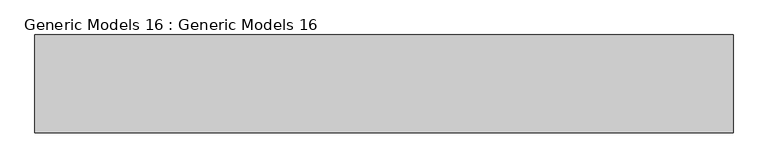
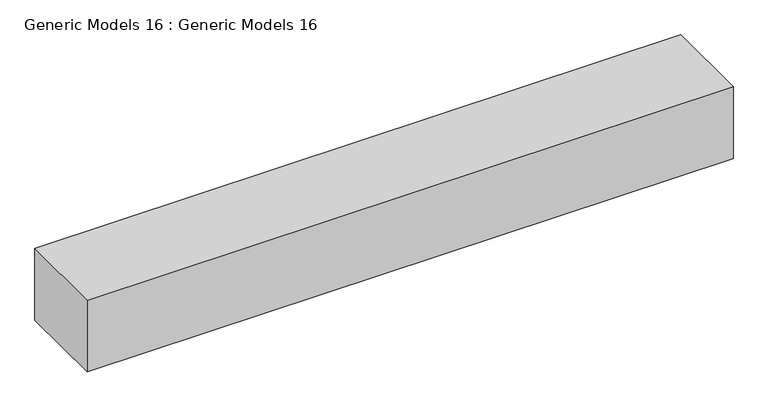
"""IFC4 building model written with IfcOpenShell, lengths in millimetres: proxy geometry, Generic Models 16 : Generic Models 16."""

from ifc_helpers import new_model, si_unit, frame, origin, place, context, project, spatial, polyline, outline, extrude, source, transform, mapped, element, save


def generic_models_16_generic_models_16_89dc7be6(model_context):
    return source(origin(), model_context, "Body", "SweptSolid", [
        extrude(outline(polyline([(3308.0370151, -3927.8342514), (3308.0370151, -4537.4342514), (-1049.2135668, -4537.4342514), (-1049.2135668, -3927.8342514), (3308.0370151, -3927.8342514)])), frame((0.0, 0.0, 28647.6913055), z_axis=(0.0, 0.0, 1.0), x_axis=(1.0, 0.0, 0.0)), (0.0, 0.0, 1.0), 511.7475113),
    ])


if __name__ == "__main__":
    model = new_model("IFC4")
    model_context = context("Model", 3, world=origin())
    ifc_project = project(units=[si_unit("LENGTHUNIT", "METRE", prefix="MILLI")], contexts=[model_context])
    site = spatial("IfcSite", under=ifc_project)
    building = spatial("IfcBuilding", under=site)
    placement = place(None, origin())
    generic_models_16_generic_models_16_shape = generic_models_16_generic_models_16_89dc7be6(model_context)
    element("IfcBuildingElementProxy", 1, Name="Generic Models 16 : Generic Models 16", ObjectType="Generic Models 16 : Generic Models 16", at=placement, inside=building, context=model_context, shape_type="MappedRepresentation", body=[
        mapped(generic_models_16_generic_models_16_shape, transform((0.0, 0.0, 0.0), x_axis=(1.0, 0.0, 0.0), y_axis=(0.0, 1.0, 0.0), z_axis=(0.0, 0.0, 1.0))),
    ])
    save(model, "model.ifc")
